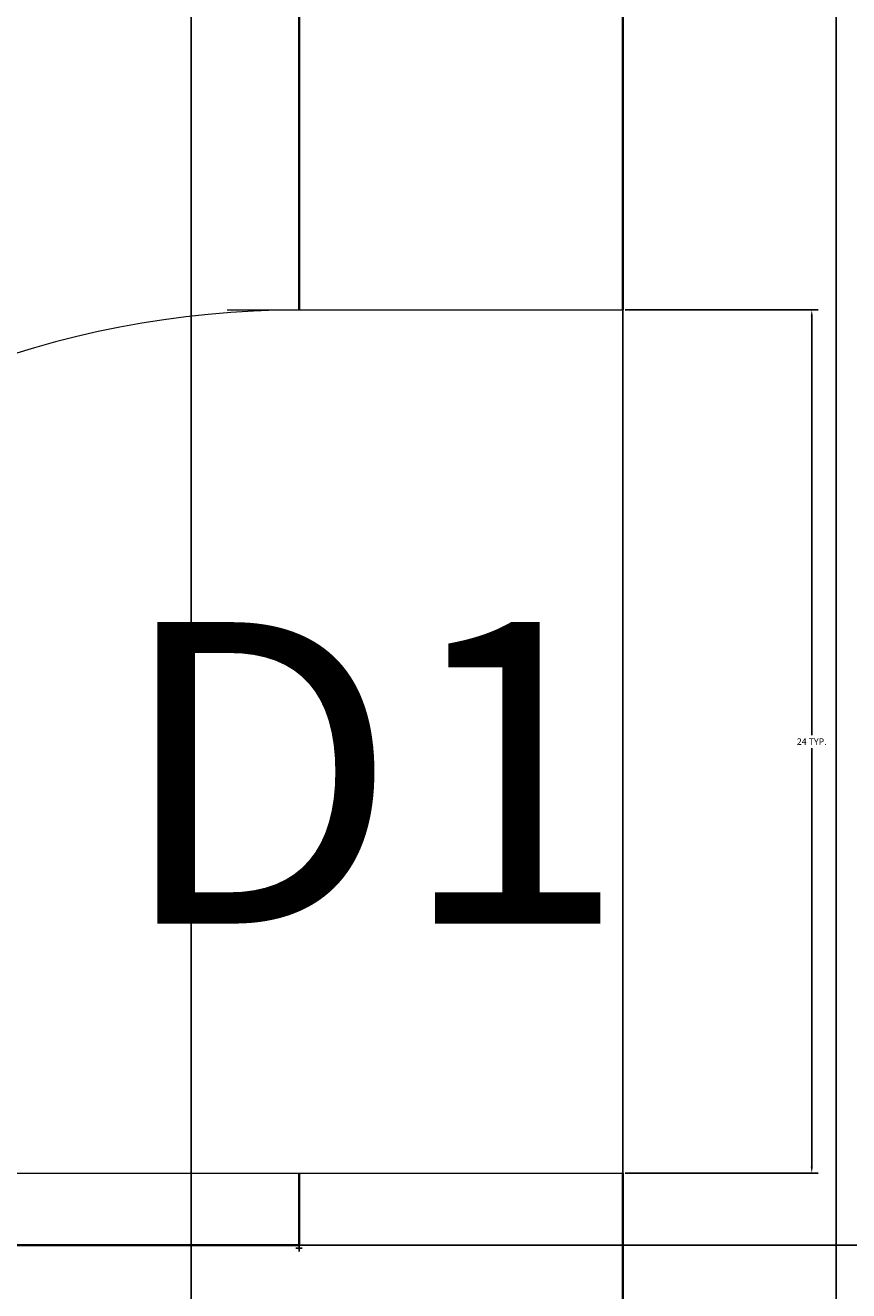
# Model space of a CAD drawing. Units: feet. Extents: x 1654 to 2985, y 1348 to 2230.
# Tile 10 of 53: x 1991 to 2014, y 1573 to 1608. Entities that reach past the tile are written whole.
import ezdxf

# ---------------------------------------------------------------- set-up
doc = ezdxf.new("R2010")
doc.units = ezdxf.units.FT
for name, color, linetype, lineweight in [('A-ANNO-DIMS', 2, 'Continuous', 18), ('A-ANNO-TEXT', 7, 'Continuous', 18), ('A-DOOR', 3, 'Continuous', 18), ('A-WALL', 7, 'Continuous', 35)]:
    doc.layers.add(name, color=color, linetype=linetype, lineweight=lineweight)
doc.styles.get("Standard").update_dxf_attribs({"font": 'arial.ttf'})
doc.dimstyles.get("Standard").update_dxf_attribs({"dimtxt": 0.18, "dimasz": 0.18, "dimexe": 0.18, "dimexo": 0.0625, "dimgap": 0.09, "dimtad": 0, "dimtih": 1, "dimtoh": 1, "dimdec": 4, "dimzin": 0, "dimdsep": 46, "dimtxsty": 'Standard', "dimcen": 0.09, "dimadec": 0, "dimazin": 0, "dimtfac": 1, "dimtdec": 4, "dimtofl": 0, "dimtmove": 0, "dimatfit": 3, "dimfxl": 1, "dimtolj": 1, "dimtzin": 0, "dimarcsym": 0})

# ---------------------------------------------------------------- blocks, each defined once
blk = doc.blocks.new('DOOR-GUEST-ENTRY')
for p, q in [((-2, 26.083), (9, 26.083)), ((-26, 2.083), (9, 2.083))]:
    blk.add_line(p, q)
blk.add_arc((0, 0), 26.083, 90, 175.4188)
blk = doc.blocks.new('*D30')
at = {"layer": 'A-ANNO-DIMS', "color": 0, "lineweight": -2, "transparency": 16777216}
for p, q in [((1973.092, 1576.192), (1973.092, 1570.825)), ((2008.092, 1576.192), (2008.092, 1570.825)), ((1973.272, 1571.005), (1989.137, 1571.005)), ((2007.912, 1571.005), (1992.048, 1571.005))]:
    blk.add_line(p, q, dxfattribs=at)
at = {"layer": 'A-ANNO-DIMS', "color": 0, "transparency": 16777216}
for points in [[(1973.272, 1571.035), (1973.272, 1570.975), (1973.092, 1571.005)], [(2007.912, 1571.035), (2007.912, 1570.975), (2008.092, 1571.005)]]:
    blk.add_solid(points, dxfattribs=at)
at = {"layer": 'Defpoints', "color": 0, "transparency": 16777216}
for p in [(1973.092, 1576.255), (2008.092, 1576.255), (2008.092, 1571.005)]:
    blk.add_point(p, dxfattribs=at)
at = {"layer": 'A-ANNO-DIMS', "color": 0, "transparency": 16777216, "insert": (1990.592, 1571.005), "char_height": 0.18, "attachment_point": 5}
blk.add_mtext('\\A1;GUEST ENTRY 35 TYP.', dxfattribs=at)
blk = doc.blocks.new('*D31')
at = {"layer": 'A-ANNO-DIMS', "color": 0, "lineweight": -2, "transparency": 16777216}
for p, q in [((2008.155, 1600.255), (2013.522, 1600.255)), ((2013.342, 1600.075), (2013.342, 1588.435)), ((2013.342, 1576.435), (2013.342, 1588.074)), ((2008.155, 1576.255), (2013.522, 1576.255))]:
    blk.add_line(p, q, dxfattribs=at)
at = {"layer": 'A-ANNO-DIMS', "color": 0, "transparency": 16777216}
for points in [[(2013.312, 1600.075), (2013.372, 1600.075), (2013.342, 1600.255)], [(2013.312, 1576.435), (2013.372, 1576.435), (2013.342, 1576.255)]]:
    blk.add_solid(points, dxfattribs=at)
at = {"layer": 'Defpoints', "color": 0, "transparency": 16777216}
for p in [(2008.092, 1600.255), (2013.342, 1600.255), (2008.092, 1576.255)]:
    blk.add_point(p, dxfattribs=at)
at = {"layer": 'A-ANNO-DIMS', "color": 0, "transparency": 16777216, "insert": (2013.342, 1588.255), "char_height": 0.18, "attachment_point": 5}
blk.add_mtext('\\A1;24 TYP.', dxfattribs=at)
blk = doc.blocks.new('*D90')
at = {"layer": 'A-ANNO-DIMS', "color": 0, "lineweight": -2, "transparency": 16777216}
for p, q in [((1852.155, 1641.187), (2242.272, 1641.187)), ((2242.092, 1641.007), (2242.092, 1607.903)), ((2242.092, 1574.435), (2242.092, 1607.539)), ((1852.155, 1574.255), (2242.272, 1574.255))]:
    blk.add_line(p, q, dxfattribs=at)
at = {"layer": 'A-ANNO-DIMS', "color": 0, "transparency": 16777216}
for points in [[(2242.062, 1641.007), (2242.122, 1641.007), (2242.092, 1641.187)], [(2242.062, 1574.435), (2242.122, 1574.435), (2242.092, 1574.255)]]:
    blk.add_solid(points, dxfattribs=at)
at = {"layer": 'Defpoints', "color": 0, "transparency": 16777216}
for p in [(1852.092, 1641.187), (2242.092, 1641.187), (1852.092, 1574.255)]:
    blk.add_point(p, dxfattribs=at)
at = {"layer": 'A-ANNO-DIMS', "color": 0, "transparency": 16777216, "insert": (2242.092, 1607.721), "char_height": 0.18, "attachment_point": 5}
blk.add_mtext('\\A1;66.93', dxfattribs=at)
blk = doc.blocks.new('*D101')
at = {"layer": 'A-ANNO-DIMS', "color": 0, "lineweight": -2, "transparency": 16777216}
for p, q in [((1996.092, 2039.192), (1996.092, 1534.075)), ((2014.016, 2039.192), (2014.016, 1534.075)), ((1996.272, 1534.255), (2004.599, 1534.255)), ((2013.836, 1534.255), (2005.509, 1534.255))]:
    blk.add_line(p, q, dxfattribs=at)
at = {"layer": 'A-ANNO-DIMS', "color": 0, "transparency": 16777216}
for points in [[(1996.272, 1534.285), (1996.272, 1534.225), (1996.092, 1534.255)], [(2013.836, 1534.285), (2013.836, 1534.225), (2014.016, 1534.255)]]:
    blk.add_solid(points, dxfattribs=at)
at = {"layer": 'Defpoints', "color": 0, "transparency": 16777216}
for p in [(1996.092, 2039.255), (2014.016, 2039.255), (2014.016, 1534.255)]:
    blk.add_point(p, dxfattribs=at)
at = {"layer": 'A-ANNO-DIMS', "color": 0, "transparency": 16777216, "insert": (2005.054, 1534.255), "char_height": 0.18, "attachment_point": 5}
blk.add_mtext('\\A1;17.924', dxfattribs=at)
blk = doc.blocks.new('*D102')
at = {"layer": 'A-ANNO-DIMS', "color": 0, "lineweight": -2, "transparency": 16777216}
for p, q in [((2008.092, 1742.192), (2008.092, 1534.075)), ((2019.757, 1742.192), (2019.757, 1534.075)), ((2008.272, 1534.255), (2013.47, 1534.255)), ((2019.577, 1534.255), (2014.379, 1534.255))]:
    blk.add_line(p, q, dxfattribs=at)
at = {"layer": 'A-ANNO-DIMS', "color": 0, "transparency": 16777216}
for points in [[(2008.272, 1534.285), (2008.272, 1534.225), (2008.092, 1534.255)], [(2019.577, 1534.285), (2019.577, 1534.225), (2019.757, 1534.255)]]:
    blk.add_solid(points, dxfattribs=at)
at = {"layer": 'Defpoints', "color": 0, "transparency": 16777216}
for p in [(2008.092, 1742.255), (2019.757, 1742.255), (2019.757, 1534.255)]:
    blk.add_point(p, dxfattribs=at)
at = {"layer": 'A-ANNO-DIMS', "color": 0, "transparency": 16777216, "insert": (2013.925, 1534.255), "char_height": 0.18, "attachment_point": 5}
blk.add_mtext('\\A1;11.664', dxfattribs=at)
blk = doc.blocks.new('*D105')
at = {"layer": 'A-ANNO-DIMS', "color": 0, "lineweight": -2, "transparency": 16777216}
for p, q in [((1970.606, 1604.838), (1970.786, 1604.838)), ((1970.786, 1604.838), (1981.279, 1593.47)), ((1999.002, 1574.172), (1999.182, 1574.172)), ((1999.092, 1574.082), (1999.092, 1574.262))]:
    blk.add_line(p, q, dxfattribs=at)
at = {"layer": 'A-ANNO-DIMS', "color": 0, "transparency": 16777216}
blk.add_solid([(1981.301, 1593.491), (1981.257, 1593.45), (1981.401, 1593.338)], dxfattribs=at)
at = {"layer": 'Defpoints', "color": 0, "transparency": 16777216}
for p in [(1981.401, 1593.338), (1999.092, 1574.172)]:
    blk.add_point(p, dxfattribs=at)
at = {"layer": 'A-ANNO-DIMS', "color": 0, "transparency": 16777216, "insert": (1970.056, 1604.838), "char_height": 0.18, "attachment_point": 5}
blk.add_mtext('\\A1;R26.083', dxfattribs=at)

msp = doc.modelspace()

# ---------------------------------------------------------------- linework, layer by layer
at = {"layer": 'A-WALL'}
for p, q in [((1999.0924, 1600.2549), (1999.0924, 1742.2549)), ((2008.0924, 1600.2549), (2008.0924, 1661.2549)), ((1999.0924, 1574.2549), (1999.0924, 1576.2549)), ((2008.0924, 1565.2549), (2008.0924, 1576.2549)), ((1852.0924, 1574.2549), (1999.0924, 1574.2549))]:
    msp.add_line(p, q, dxfattribs=at)

# ---------------------------------------------------------------- block references
at = {"layer": 'A-DOOR'}
msp.add_blockref('DOOR-GUEST-ENTRY', (1999.0924, 1574.1716), dxfattribs=at)

# ---------------------------------------------------------------- texts
at = {"layer": 'A-ANNO-TEXT'}
msp.add_text('D1', height=8.38114, dxfattribs=at).set_placement((1993.9957, 1583.1952))

# ---------------------------------------------------------------- dimensions: what is measured, and where the dimension line sits
at = {"layer": 'A-ANNO-DIMS'}
for base, p1, p2, picture, middle in [((2014.016, 1534.2549), (1996.0924, 2039.2549), (2014.016, 2039.2549), '*D101', (2005.0542, 1534.2549)), ((2019.7567, 1534.2549), (2008.0924, 1742.2549), (2019.7567, 1742.2549), '*D102', (2013.9246, 1534.2549))]:
    dim = msp.add_linear_dim(base=base, p1=p1, p2=p2, dimstyle='Standard', override={"dimdec": 3, "dimlfac": 1, "dimrnd": 0, "dimzin": 0, "dimdsep": 46, "dimlunit": 2}, dxfattribs=at)
    dim.commit()
    dim.dimension.update_dxf_attribs({"geometry": picture, "text_midpoint": middle})
dim = msp.add_linear_dim(base=(2242.0924, 1641.187), p1=(1852.0924, 1574.2549), p2=(1852.0924, 1641.187), angle=90, dimstyle='Standard', override={"dimdec": 2, "dimlfac": 1, "dimrnd": 0, "dimzin": 0, "dimdsep": 46, "dimlunit": 2}, dxfattribs=at)
dim.commit()
dim.dimension.update_dxf_attribs({"geometry": '*D90', "text_midpoint": (2242.0924, 1607.721)})
dim = msp.add_radius_dim(center=(1999.0924, 1574.1716), mpoint=(1981.401, 1593.338), dimstyle='Standard', override={"dimdec": 3, "dimlfac": 1, "dimrnd": 0, "dimzin": 0, "dimdsep": 46, "dimlunit": 2}, dxfattribs=at)
dim.commit()
dim.dimension.update_dxf_attribs({"geometry": '*D105', "text_midpoint": (1970.0563, 1604.8379), "dimtype": 164})
dim = msp.add_linear_dim(base=(2013.3424, 1600.2549), p1=(2008.0924, 1576.2549), p2=(2008.0924, 1600.2549), angle=90, text='<> TYP.', dimstyle='Standard', override={"dimdec": 0, "dimlfac": 1, "dimrnd": 0, "dimzin": 0, "dimdsep": 46, "dimlunit": 2}, dxfattribs=at)
dim.commit()
dim.dimension.update_dxf_attribs({"geometry": '*D31', "text_midpoint": (2013.3424, 1588.2549)})
dim = msp.add_linear_dim(base=(2008.0924, 1571.0049), p1=(1973.0924, 1576.2549), p2=(2008.0924, 1576.2549), text='GUEST ENTRY <> TYP.', dimstyle='Standard', override={"dimdec": 0, "dimlfac": 1, "dimrnd": 0, "dimzin": 0, "dimdsep": 46, "dimlunit": 2}, dxfattribs=at)
dim.commit()
dim.dimension.update_dxf_attribs({"geometry": '*D30', "text_midpoint": (1990.5924, 1571.0049)})

doc.saveas('drawing.dxf')
